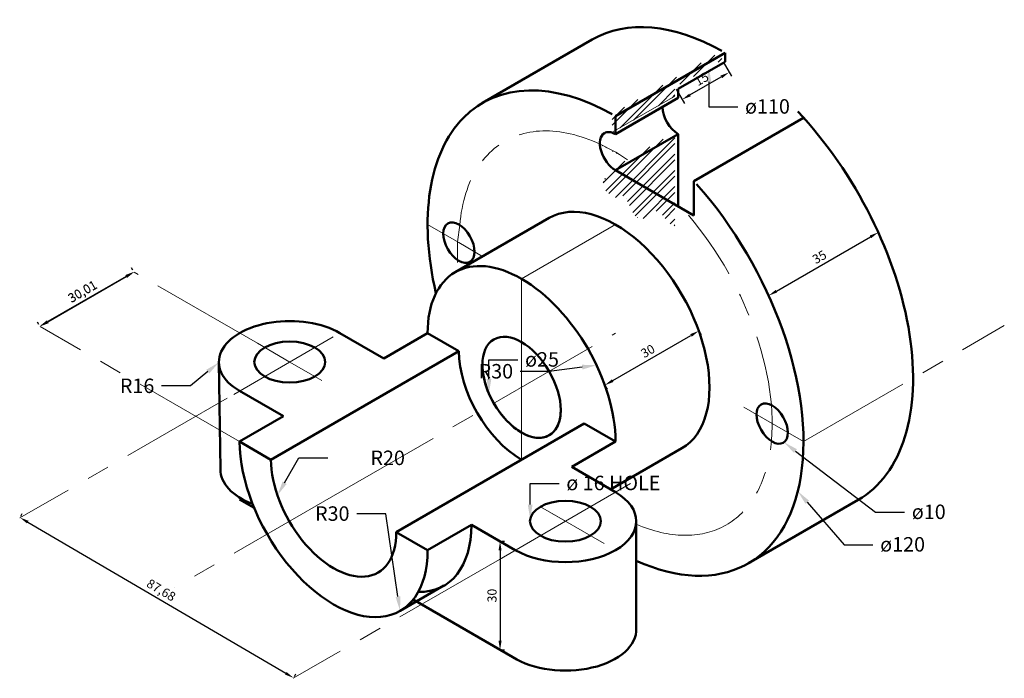
# Model space of a CAD drawing. Units: millimetres. Extents: x 2830 to 3102, y 1462 to 1644.
import ezdxf
from ezdxf import colors
from ezdxf.entities.mleader import LeaderData, LeaderLine
from ezdxf.math import Vec2, Vec3

# ---------------------------------------------------------------- set-up
doc = ezdxf.new("R2010")
doc.units = ezdxf.units.MM
doc.linetypes.add('CENTER', pattern=[50.8, 31.75, -6.35, 6.35, -6.35])
for name, color, linetype, lineweight in [('M-CNTR', 1, 'CENTER', 18), ('M-DIMS', 2, 'Continuous', 25), ('M-HATC', 8, 'Continuous', 18), ('M-OUTL', 7, 'Continuous', 50), ('M-TEXT', 3, 'Continuous', 25)]:
    doc.layers.add(name, color=color, linetype=linetype, lineweight=lineweight)
doc.styles.get("Standard").update_dxf_attribs({"font": 'arial.ttf'})
doc.dimstyles.new('ISO-25', dxfattribs={"dimtxt": 2.5, "dimasz": 2.5, "dimexe": 1.25, "dimexo": 0.625, "dimtad": 1, "dimtxsty": 'Standard', "dimcen": 2.5, "dimadec": 0, "dimazin": 0, "dimtfac": 1, "dimtmove": 0, "dimatfit": 3, "dimfxl": 1, "dimarcsym": 0})
pattern_1 = [(45, (0, 0), (-2.245064, 2.245064), []), (45, (0, 1.5875), (-2.245064, 2.245064), [])]

# ---------------------------------------------------------------- blocks, each defined once
blk = doc.blocks.new('*D1')
at = {"layer": 'Defpoints', "color": 0, "transparency": 16777216}
for p in [(2962.61, 1500.11), (2962.61, 1470.11), (2962.61, 1470.11)]:
    blk.add_point(p, dxfattribs=at)
at = {"layer": 'M-DIMS', "color": 0, "lineweight": -2, "transparency": 16777216}
for p, q in [((2963.24, 1500.11), (2963.86, 1500.11)), ((2962.61, 1497.61), (2962.61, 1472.61)), ((2963.24, 1470.11), (2963.86, 1470.11))]:
    blk.add_line(p, q, dxfattribs=at)
at = {"layer": 'M-DIMS', "color": 0, "transparency": 16777216}
for points in [[(2962.19, 1497.61), (2963.03, 1497.61), (2962.61, 1500.11)], [(2962.19, 1472.61), (2963.03, 1472.61), (2962.61, 1470.11)]]:
    blk.add_solid(points, dxfattribs=at)
at = {"layer": 'M-DIMS', "color": 0, "transparency": 16777216, "insert": (2960.71, 1485.11), "char_height": 2.5, "attachment_point": 5, "rotation": 90}
blk.add_mtext('30', dxfattribs=at)
blk = doc.blocks.new('*D2')
at = {"layer": 'Defpoints', "color": 0, "transparency": 16777216}
for p in [(3017.56, 1558.28), (3017.56, 1558.28), (2991.58, 1543.28)]:
    blk.add_point(p, dxfattribs=at)
at = {"layer": 'M-DIMS', "color": 0, "lineweight": -2, "transparency": 16777216}
for p, q in [((3017.88, 1557.74), (3018.19, 1557.2)), ((2993.75, 1544.53), (3015.4, 1557.03)), ((2991.89, 1542.74), (2992.21, 1542.2))]:
    blk.add_line(p, q, dxfattribs=at)
at = {"layer": 'M-DIMS', "color": 0, "transparency": 16777216}
for points in [[(3015.19, 1557.39), (3015.61, 1556.67), (3017.56, 1558.28)], [(2993.54, 1544.89), (2993.96, 1544.17), (2991.58, 1543.28)]]:
    blk.add_solid(points, dxfattribs=at)
at = {"layer": 'M-DIMS', "color": 0, "transparency": 16777216, "insert": (3003.62, 1552.43), "char_height": 2.5, "attachment_point": 5, "rotation": 30}
blk.add_mtext('30', dxfattribs=at)
blk = doc.blocks.new('*D3')
at = {"layer": 'Defpoints', "color": 0, "transparency": 16777216}
for p in [(3023.96, 1633.18), (3025.94, 1629.75), (3010.97, 1625.68)]:
    blk.add_point(p, dxfattribs=at)
at = {"layer": 'M-DIMS', "color": 0, "lineweight": -2, "transparency": 16777216}
for p, q in [((3024.28, 1632.64), (3026.57, 1628.66)), ((3015.12, 1623.5), (3023.78, 1628.5)), ((3011.29, 1625.14), (3013.58, 1621.16))]:
    blk.add_line(p, q, dxfattribs=at)
at = {"layer": 'M-DIMS', "color": 0, "transparency": 16777216}
for points in [[(3023.57, 1628.86), (3023.99, 1628.14), (3025.94, 1629.75)], [(3014.91, 1623.86), (3015.33, 1623.14), (3012.95, 1622.25)]]:
    blk.add_solid(points, dxfattribs=at)
at = {"layer": 'M-DIMS', "color": 0, "transparency": 16777216, "insert": (3018.5, 1627.64), "char_height": 2.5, "attachment_point": 5, "rotation": 30}
blk.add_mtext('15', dxfattribs=at)
blk = doc.blocks.new('*D4')
at = {"layer": 'Defpoints', "color": 0, "transparency": 16777216}
for p in [(3067.18, 1585.53), (3067.18, 1585.53), (3036.87, 1568.03)]:
    blk.add_point(p, dxfattribs=at)
at = {"layer": 'M-DIMS', "color": 0, "lineweight": -2, "transparency": 16777216}
for p, q in [((3067.49, 1584.99), (3067.81, 1584.45)), ((3039.03, 1569.28), (3065.02, 1584.28)), ((3037.18, 1567.49), (3037.49, 1566.95))]:
    blk.add_line(p, q, dxfattribs=at)
at = {"layer": 'M-DIMS', "color": 0, "transparency": 16777216}
for points in [[(3064.81, 1584.64), (3065.22, 1583.92), (3067.18, 1585.53)], [(3038.83, 1569.64), (3039.24, 1568.92), (3036.87, 1568.03)]]:
    blk.add_solid(points, dxfattribs=at)
at = {"layer": 'M-DIMS', "color": 0, "transparency": 16777216, "insert": (3051.07, 1578.43), "char_height": 2.5, "attachment_point": 5, "rotation": 30}
blk.add_mtext('35', dxfattribs=at)
blk = doc.blocks.new('*D5')
at = {"layer": 'Defpoints', "color": 0, "transparency": 16777216}
for p in [(2829.8, 1506.56), (2905.45, 1462.24), (2905.52, 1462.36)]:
    blk.add_point(p, dxfattribs=at)
at = {"layer": 'M-DIMS', "color": 0, "lineweight": -2, "transparency": 16777216}
for p, q in [((2830.12, 1507.1), (2830.5, 1507.76)), ((2832.03, 1505.42), (2903.37, 1463.63)), ((2905.77, 1462.78), (2906.16, 1463.44))]:
    blk.add_line(p, q, dxfattribs=at)
at = {"layer": 'M-DIMS', "color": 0, "transparency": 16777216}
for points in [[(2832.24, 1505.78), (2831.82, 1505.06), (2829.87, 1506.69)], [(2903.58, 1463.99), (2903.16, 1463.27), (2905.52, 1462.36)]]:
    blk.add_solid(points, dxfattribs=at)
at = {"layer": 'M-DIMS', "color": 0, "transparency": 16777216, "insert": (2868.77, 1486.36), "char_height": 2.5, "attachment_point": 5, "rotation": 329.6353}
blk.add_mtext('87,68', dxfattribs=at)
blk = doc.blocks.new('*D6')
at = {"layer": 'Defpoints', "color": 0, "transparency": 16777216}
for p in [(2829.8, 1506.56), (2905.45, 1462.24), (2905.52, 1462.36)]:
    blk.add_point(p, dxfattribs=at)
at = {"layer": 'M-DIMS', "color": 0, "lineweight": -2, "transparency": 16777216}
for p, q in [((2830.12, 1507.1), (2830.5, 1507.76)), ((2832.03, 1505.42), (2903.37, 1463.63)), ((2905.77, 1462.78), (2906.16, 1463.44))]:
    blk.add_line(p, q, dxfattribs=at)
at = {"layer": 'M-DIMS', "color": 0, "transparency": 16777216}
for points in [[(2832.24, 1505.78), (2831.82, 1505.06), (2829.87, 1506.69)], [(2903.58, 1463.99), (2903.16, 1463.27), (2905.52, 1462.36)]]:
    blk.add_solid(points, dxfattribs=at)
at = {"layer": 'M-DIMS', "color": 0, "transparency": 16777216, "insert": (2868.77, 1486.36), "char_height": 2.5, "attachment_point": 5, "rotation": 329.6353}
blk.add_mtext('87,68', dxfattribs=at)
blk = doc.blocks.new('*D7')
at = {"layer": 'Defpoints', "color": 0, "transparency": 16777216}
for p in [(2861.42, 1574.53), (2835.38, 1559.61), (2835.43, 1559.53)]:
    blk.add_point(p, dxfattribs=at)
at = {"layer": 'M-DIMS', "color": 0, "lineweight": -2, "transparency": 16777216}
for p, q in [((2861.1, 1575.08), (2860.74, 1575.7)), ((2859.2, 1573.36), (2837.55, 1560.86)), ((2835.11, 1560.07), (2834.76, 1560.69))]:
    blk.add_line(p, q, dxfattribs=at)
at = {"layer": 'M-DIMS', "color": 0, "transparency": 16777216}
for points in [[(2859, 1573.72), (2859.41, 1573), (2861.37, 1574.61)], [(2837.34, 1561.22), (2837.76, 1560.5), (2835.38, 1559.61)]]:
    blk.add_solid(points, dxfattribs=at)
at = {"layer": 'M-DIMS', "color": 0, "transparency": 16777216, "insert": (2847.31, 1568.95), "char_height": 2.5, "attachment_point": 5, "rotation": 30}
blk.add_mtext('30,01', dxfattribs=at)
blk = doc.blocks.new('*D8')
at = {"layer": 'Defpoints', "color": 0, "transparency": 16777216}
for p in [(2861.42, 1574.53), (2861.42, 1574.53), (2835.43, 1559.53)]:
    blk.add_point(p, dxfattribs=at)
at = {"layer": 'M-DIMS', "color": 0, "lineweight": -2, "transparency": 16777216}
for p, q in [((2861.1, 1575.08), (2860.79, 1575.62)), ((2837.59, 1560.78), (2859.25, 1573.28)), ((2835.11, 1560.07), (2834.8, 1560.61))]:
    blk.add_line(p, q, dxfattribs=at)
at = {"layer": 'M-DIMS', "color": 0, "transparency": 16777216}
for points in [[(2859.04, 1573.65), (2859.46, 1572.92), (2861.42, 1574.53)], [(2837.38, 1561.14), (2837.8, 1560.42), (2835.43, 1559.53)]]:
    blk.add_solid(points, dxfattribs=at)
at = {"layer": 'M-DIMS', "color": 0, "transparency": 16777216, "insert": (2847.36, 1568.87), "char_height": 2.5, "attachment_point": 5, "rotation": 30}
blk.add_mtext('30,01', dxfattribs=at)

msp = doc.modelspace()

# ---------------------------------------------------------------- hatches: boundary and pattern name
at = {"layer": 'M-HATC'}
h = msp.add_hatch(dxfattribs=at)
h.set_pattern_fill('STEEL', color=256)
h.set_pattern_definition(pattern_1)
h.paths.add_polyline_path([(3010.973, 1623.178), (3010.973, 1625.678), (3023.963, 1633.178), (3023.963, 1635.679), (2993.652, 1618.179), (2993.652, 1613.177)])
h = msp.add_hatch(dxfattribs=at)
h.set_pattern_fill('STEEL', color=256)
h.set_pattern_definition(pattern_1)
h.paths.add_polyline_path([(2996.27, 1595.472), (2996.241, 1595.455), (2996.172, 1595.411), (2996.221, 1595.442)])
h.paths.add_polyline_path([(3006.737, 1619.58), (3006.744, 1619.541), (3006.74, 1619.567), (3006.735, 1619.593), (3006.731, 1619.619)])
h.paths.add_polyline_path([(2996.46, 1595.577), (2996.438, 1595.567), (2996.413, 1595.554)])
h.paths.add_polyline_path([(2996.552, 1595.616), (2996.531, 1595.609), (2996.506, 1595.598)])
h.paths.add_polyline_path([(3006.721, 1619.684), (3006.727, 1619.645), (3006.723, 1619.671), (3006.719, 1619.697), (3006.715, 1619.723)])
h.paths.add_polyline_path([(3006.755, 1619.476), (3006.763, 1619.436), (3006.758, 1619.462), (3006.753, 1619.489), (3006.749, 1619.515)])
h.paths.add_polyline_path([(2996.366, 1595.528), (2996.345, 1595.517), (2996.318, 1595.501)])
h.paths.add_polyline_path([(2996.643, 1595.643), (2996.622, 1595.639), (2996.598, 1595.631)])
h.paths.add_polyline_path([(3006.706, 1619.788), (3006.711, 1619.749), (3006.708, 1619.775), (3006.704, 1619.801), (3006.701, 1619.827)])
h.paths.add_polyline_path([(3006.775, 1619.37), (3006.783, 1619.331), (3006.778, 1619.357), (3006.773, 1619.384), (3006.768, 1619.41)])
h.paths.add_polyline_path([(3006.692, 1619.891), (3006.697, 1619.852), (3006.694, 1619.878), (3006.691, 1619.904), (3006.688, 1619.929)])
h.paths.add_polyline_path([(2996.734, 1595.655), (2996.712, 1595.655), (2996.689, 1595.651)])
h.paths.add_polyline_path([(3006.68, 1619.993), (3006.685, 1619.955), (3006.682, 1619.981), (3006.679, 1620.006), (3006.677, 1620.032)])
h.paths.add_polyline_path([(3006.797, 1619.265), (3006.805, 1619.225), (3006.8, 1619.252), (3006.794, 1619.278), (3006.789, 1619.304)])
h.paths.add_polyline_path([(3006.67, 1620.095), (3006.674, 1620.057), (3006.671, 1620.082), (3006.669, 1620.108), (3006.667, 1620.133)])
h.paths.add_polyline_path([(2996.824, 1595.65), (2996.802, 1595.655), (2996.779, 1595.655)])
h.paths.add_polyline_path([(3006.661, 1620.196), (3006.665, 1620.158), (3006.663, 1620.183), (3006.661, 1620.209), (3006.659, 1620.234)])
h.paths.add_polyline_path([(3006.819, 1619.159), (3006.829, 1619.119), (3006.823, 1619.146), (3006.817, 1619.172), (3006.811, 1619.199)])
h.paths.add_polyline_path([(3006.654, 1620.296), (3006.657, 1620.259), (3006.655, 1620.284), (3006.654, 1620.309), (3006.652, 1620.334)])
h.paths.add_polyline_path([(2996.913, 1595.625), (2996.892, 1595.635), (2996.869, 1595.64)])
h.paths.add_polyline_path([(3006.649, 1620.396), (3006.651, 1620.358), (3006.65, 1620.383), (3006.649, 1620.408), (3006.648, 1620.433)])
h.paths.add_polyline_path([(3006.843, 1619.057), (3006.847, 1619.039), (3006.841, 1619.066), (3006.835, 1619.092)])
h.paths.add_polyline_path([(3006.645, 1620.494), (3006.647, 1620.457), (3006.646, 1620.482), (3006.645, 1620.507), (3006.644, 1620.531)])
h.paths.add_polyline_path([(2997.003, 1595.579), (2996.981, 1595.595), (2996.958, 1595.605)])
h.paths.add_polyline_path([(3006.643, 1620.592), (3006.644, 1620.555), (3006.643, 1620.58), (3006.643, 1620.604), (3006.643, 1620.628)])
h.paths.add_polyline_path([(2997.094, 1595.508), (2997.072, 1595.53), (2997.049, 1595.547)])
h.paths.add_polyline_path([(3006.642, 1620.677), (3006.643, 1620.653), (3006.642, 1620.677)])
h.paths.add_polyline_path([(2997.185, 1595.411), (2997.162, 1595.44), (2997.139, 1595.463)])
h = msp.add_hatch(dxfattribs=at)
h.set_pattern_fill('STARS', color=256)
edge = h.paths.add_edge_path(flags=17)
edge.add_line((3010.973, 1613.177), (2997.982, 1605.677))
edge.add_ellipse((2993.652, 1608.177), major_axis=(3.062, -5.303), ratio=0.5773503, start_angle=28.55472, end_angle=30, ccw=False)
edge.add_ellipse((2994.538, 1557.676), major_axis=(30.619, -53.033), ratio=0.5773503, start_angle=146.03159, end_angle=155.64724, ccw=False)
edge.add_line((2997.863, 1605.608), (2993.652, 1603.177))
edge.add_spline(control_points=[(2993.652, 1603.177), (2989.631, 1598.94), (2992.844, 1596.003), (2995.663, 1594.375), (2997.082, 1596.832), (2998.786, 1591.134), (3001.829, 1587.953), (3006.458, 1593.12), (3008.118, 1588.818), (3010.248, 1587.415), (3010.973, 1587.275)], knot_values=[0, 0, 0, 0, 1, 2, 3, 4, 5, 6, 7, 7.4719642, 7.4719642, 7.4719642, 7.4719642], degree=3, periodic=0)
edge.add_line((3010.973, 1587.275), (3010.973, 1613.177))
edge = h.paths.add_edge_path(flags=17)
edge.add_line((3010.973, 1613.177), (2997.982, 1605.677))
edge.add_ellipse((2993.652, 1608.177), major_axis=(3.062, -5.303), ratio=0.5773503, start_angle=29.2721, end_angle=30, ccw=False)
edge.add_ellipse((2994.538, 1557.676), major_axis=(30.619, -53.033), ratio=0.5773503, start_angle=146.03159, end_angle=155.64724, ccw=False)
edge.add_line((2997.863, 1605.608), (2993.652, 1603.177))
edge.add_line((2993.652, 1603.177), (2991.105, 1598.999))
edge.add_line((2991.105, 1598.999), (2992.044, 1596.855))
edge.add_line((2992.044, 1596.855), (2993.629, 1595.653))
edge.add_line((2993.629, 1595.653), (2994.875, 1595.072))
edge.add_line((2994.875, 1595.072), (2995.823, 1595.202))
edge.add_line((2995.823, 1595.202), (2995.963, 1595.281))
edge.add_spline(control_points=[(2995.963, 1595.281), (2996.181, 1595.411), (2996.378, 1595.557), (2996.568, 1595.622)], knot_values=[2.2737758, 2.2737758, 2.2737758, 2.2737758, 2.6371638, 2.6371638, 2.6371638, 2.6371638], degree=3, periodic=0)
edge.add_line((2996.534, 1595.637), (2996.568, 1595.622))
edge.add_spline(control_points=[(2996.568, 1595.622), (2996.758, 1595.686), (2996.979, 1595.665), (2997.21, 1595.382), (2997.25, 1595.326)], knot_values=[2.6371638, 2.6371638, 2.6371638, 2.6371638, 3, 3.0766912, 3.0766912, 3.0766912, 3.0766912], degree=3, periodic=0)
edge.add_spline(control_points=[(2997.25, 1595.326), (2997.483, 1595.001), (2997.727, 1594.44), (2997.998, 1593.794)], knot_values=[3.0766912, 3.0766912, 3.0766912, 3.0766912, 3.5162185, 3.5162185, 3.5162185, 3.5162185], degree=3, periodic=0)
edge.add_line((2997.998, 1593.794), (2998.905, 1591.752))
edge.add_line((2998.905, 1591.752), (3000.054, 1590.055))
edge.add_line((3000.054, 1590.055), (3001.481, 1589.29))
edge.add_line((3001.481, 1589.29), (3003.191, 1589.866))
edge.add_line((3003.191, 1589.866), (3003.643, 1590.164))
edge.add_spline(control_points=[(3003.643, 1590.164), (3004.098, 1590.474), (3004.552, 1590.805), (3004.981, 1591.044)], knot_values=[5.3837355, 5.3837355, 5.3837355, 5.3837355, 5.713855, 5.713855, 5.713855, 5.713855], degree=3, periodic=0)
edge.add_spline(control_points=[(3004.981, 1591.044), (3005.353, 1591.252), (3005.895, 1591.466), (3006.352, 1591.345), (3006.505, 1591.27)], knot_values=[5.713855, 5.713855, 5.713855, 5.713855, 6, 6.1533823, 6.1533823, 6.1533823, 6.1533823], degree=3, periodic=0)
edge.add_spline(control_points=[(3006.505, 1591.27), (3006.943, 1591.056), (3007.325, 1590.575), (3007.733, 1590.019)], knot_values=[6.1533823, 6.1533823, 6.1533823, 6.1533823, 6.5929096, 6.5929096, 6.5929096, 6.5929096], degree=3, periodic=0)
edge.add_line((3007.733, 1590.019), (3009.118, 1588.318))
edge.add_line((3009.118, 1588.318), (3010.973, 1587.275))
edge.add_line((3010.973, 1587.275), (3010.973, 1613.177))
h = msp.add_hatch(dxfattribs=at)
h.set_pattern_fill('STEEL', color=256)
h.set_pattern_definition(pattern_1)
edge = h.paths.add_edge_path()
edge.add_line((3010.973, 1613.177), (2997.982, 1605.677))
edge.add_ellipse((2993.652, 1608.177), major_axis=(3.062, -5.303), ratio=0.5773503, start_angle=28.55472, end_angle=30, ccw=False)
edge.add_ellipse((2994.538, 1557.676), major_axis=(30.619, -53.033), ratio=0.5773503, start_angle=146.03159, end_angle=155.64724, ccw=False)
edge.add_line((2997.863, 1605.608), (2993.652, 1603.177))
edge.add_spline(control_points=[(2993.652, 1603.177), (2989.631, 1598.94), (2992.844, 1596.003), (2995.663, 1594.375), (2997.082, 1596.832), (2998.786, 1591.134), (3001.829, 1587.953), (3006.458, 1593.12), (3008.118, 1588.818), (3010.248, 1587.415), (3010.973, 1587.275)], knot_values=[0, 0, 0, 0, 1, 2, 3, 4, 5, 6, 7, 7.4719642, 7.4719642, 7.4719642, 7.4719642], degree=3, periodic=0)
edge.add_line((3010.973, 1587.275), (3010.973, 1613.177))

# ---------------------------------------------------------------- linework, layer by layer
at = {"layer": 'M-CNTR'}
for p, q in [((3006.642, 1620.677), (3010.973, 1623.177)), ((2993.652, 1613.177), (3006.642, 1620.677)), ((2951.237, 1582.676), (2942.577, 1587.676)), ((2951.453, 1587.544), (2950.83, 1582.911)), ((2968.557, 1572.676), (2994.538, 1587.676)), ((2950.83, 1582.911), (2950.83, 1577.172)), ((2951.237, 1582.676), (2957.796, 1578.889)), ((2895.512, 1554.848), (2861.415, 1574.534)), ((2968.557, 1542.676), (2968.557, 1572.676)), ((2890.615, 1527.668), (2835.427, 1559.53)), ((2916.596, 1512.676), (2994.538, 1557.676)), ((3046.5, 1527.676), (3102.024, 1559.733)), ((2916.494, 1556.617), (2887.186, 1539.696)), ((2904.472, 1549.676), (2895.512, 1554.848)), ((2911.4, 1545.676), (2904.472, 1549.676)), ((2911.4, 1545.676), (2913.291, 1544.584)), ((2968.557, 1542.676), (2968.557, 1522.676)), ((2887.186, 1539.696), (2829.801, 1506.565)), ((3037.839, 1532.676), (3030.05, 1537.173)), ((3037.839, 1532.676), (3046.5, 1527.676)), ((2980.682, 1505.676), (2998.697, 1516.077)), ((2916.596, 1512.676), (2872.583, 1487.265)), ((2973.754, 1509.676), (2980.682, 1505.676)), ((2973.754, 1509.676), (2991.349, 1499.517)), ((2980.682, 1505.676), (2962.415, 1495.129)), ((2962.415, 1495.129), (2905.454, 1462.243))]:
    msp.add_line(p, q, dxfattribs=at)
for start_param, end_param in [(2.2793263, 3.8269491), (5.6294391, 8.1539794)]:
    msp.add_ellipse((2994.538, 1557.676), major_axis=(30.619, -53.033), ratio=0.5773503, start_param=start_param, end_param=end_param, dxfattribs=at)
at = {"layer": 'M-OUTL'}
for p, q in [((2957.796, 1621.315), (2988.107, 1638.815)), ((2988.107, 1638.815), (2957.796, 1621.315)), ((2994.538, 1617.676), (3024.849, 1635.176)), ((3024.849, 1632.676), (3024.849, 1635.176)), ((3011.859, 1625.176), (3024.849, 1632.676)), ((3011.859, 1625.176), (3011.859, 1622.676)), ((2994.538, 1612.676), (3011.859, 1622.676)), ((2994.538, 1617.676), (2994.538, 1612.676)), ((3016.189, 1599.72), (3046.5, 1617.22)), ((2994.538, 1602.676), (3011.859, 1612.676)), ((3011.859, 1612.676), (3011.859, 1592.676)), ((3016.189, 1590.176), (2994.538, 1602.676)), ((3016.189, 1599.72), (3016.189, 1590.176)), ((2950.186, 1574.495), (2976.167, 1589.495)), ((2918.328, 1557.676), (2930.452, 1550.676)), ((2930.452, 1550.676), (2942.577, 1557.676)), ((2951.237, 1552.676), (2942.577, 1557.676)), ((2899.275, 1522.676), (2951.237, 1552.676)), ((2899.275, 1522.676), (2951.237, 1552.676)), ((2885.305, 1520.062), (2884.876, 1549.581)), ((2890.615, 1541.676), (2902.74, 1534.676)), ((2890.615, 1527.676), (2902.74, 1534.676)), ((2933.916, 1502.676), (2985.878, 1532.676)), ((2985.878, 1532.676), (2994.538, 1527.676)), ((2899.275, 1522.676), (2890.615, 1527.676)), ((2982.414, 1520.676), (2994.538, 1527.676)), ((2982.414, 1520.676), (2994.538, 1527.676)), ((3012.909, 1525.856), (2993.175, 1514.462)), ((2982.414, 1520.676), (2994.538, 1513.676)), ((2894.619, 1509.365), (2890.615, 1511.676)), ((3031.281, 1494.036), (3061.591, 1511.536)), ((3000.278, 1475.676), (3000.278, 1505.676)), ((2933.916, 1502.676), (2942.577, 1497.676)), ((2942.577, 1497.676), (2933.916, 1502.676)), ((2942.577, 1497.676), (2954.701, 1504.676)), ((2942.577, 1497.676), (2954.701, 1504.676)), ((2954.701, 1504.676), (2966.825, 1497.676)), ((2934.967, 1480.856), (2947.092, 1487.856)), ((2966.144, 1468.089), (2938.584, 1484.001))]:
    msp.add_line(p, q, dxfattribs=at)
for centre, major_axis, start_param, end_param in [((3024.849, 1575.176), (36.742, -63.64), 2.3732487, 3.1415927), ((2994.538, 1557.676), (36.742, -63.64), 8.656434, 10.5088793), ((3011.859, 1617.676), (3.062, -5.303), 3.9269908, 5.4977871), ((3024.849, 1575.176), (36.742, -63.64), 0, 1.9596753), ((2994.538, 1607.676), (3.062, -5.303), 3.1415927, 5.4977871), ((2994.538, 1607.676), (3.062, -5.303), 2.3561945, 3.1415927), ((2994.538, 1557.676), (36.742, -63.64), 5.6084699, 8.1933451), ((2994.538, 1557.676), (18.371, -31.82), 0, 3.1415927), ((2968.558, 1542.676), (18.371, -31.82), 2.3561945, 3.1415927), ((2968.558, 1542.676), (18.371, -31.82), 3.1415927, 3.9269908), ((2994.538, 1557.676), (30.619, -53.033), 4.0688879, 4.0712043), ((2968.558, 1542.676), (18.371, -31.82), 0.7853982, 2.3561945), ((2904.472, 1549.676), (-19.596, 0), 3.9269908, 7.0685835), ((2968.557, 1542.676), (12.247, -21.213), 3.9269908, 5.4977871), ((2968.557, 1542.676), (7.655, -13.258), 3.9269908, 7.0685835), ((2904.899, 1519.923), (-19.596, 0), 5.4977871, 5.5291568), ((2916.596, 1512.676), (18.371, -31.82), 3.9269908, 7.0685835), ((2916.596, 1512.676), (12.247, -21.213), 3.9269908, 7.0685835), ((2904.899, 1519.923), (-19.596, 0), 6.2708926, 7.2751503), ((2980.682, 1505.676), (-19.596, 0), 0.7853982, 3.9269908), ((2928.72, 1519.676), (18.371, -31.82), 5.9468996, 7.0685835), ((2980.682, 1475.676), (-19.596, 0), 0.7349544, 3.1742786)]:
    msp.add_ellipse(centre, major_axis=major_axis, ratio=0.5773503, start_param=start_param, end_param=end_param, dxfattribs=at)
for centre, major_axis in [((2951.237, 1582.676), (3.062, -5.303)), ((2968.557, 1542.676), (7.655, -13.258)), ((2904.472, 1549.676), (-9.798, 0)), ((3037.839, 1532.676), (3.062, -5.303)), ((2980.682, 1505.676), (-9.798, 0))]:
    msp.add_ellipse(centre, major_axis=major_axis, ratio=0.5773503, dxfattribs=at)

# ---------------------------------------------------------------- dimensions: what is measured, and where the dimension line sits
at = {"layer": 'M-DIMS'}
for p1, p2, distance, picture, middle in [((3010.973, 1625.678), (3023.963, 1633.178), -3.963, '*D3', (3018.499, 1627.643)), ((3036.87, 1568.031), (3067.18, 1585.531), 0, '*D4', (3051.074, 1578.429)), ((2991.582, 1543.28), (3017.563, 1558.28), 0, '*D2', (3003.621, 1552.428)), ((2962.611, 1500.109), (2962.611, 1470.109), 0, '*D1', (2960.709, 1485.109))]:
    dim = msp.add_aligned_dim(p1=p1, p2=p2, distance=distance, dimstyle='ISO-25', override={"dimclrd": 0, "dimclre": 0, "dimclrt": 0}, dxfattribs=at)
    dim.commit()
    dim.dimension.update_dxf_attribs({"geometry": picture, "text_midpoint": middle})
for base, p1, p2, angle, picture, middle in [((2835.382, 1559.61), (2861.415, 1574.534), (2835.427, 1559.53), 210, '*D7', (2847.312, 1568.954)), ((2861.415, 1574.534), (2835.427, 1559.53), (2861.415, 1574.534), 30, '*D8', (2847.358, 1568.875)), ((2905.524, 1462.363), (2829.801, 1506.565), (2905.454, 1462.243), 329.63528, '*D5', (2868.774, 1486.36)), ((2905.524, 1462.363), (2829.801, 1506.565), (2905.454, 1462.243), 329.63528, '*D6', (2868.774, 1486.36))]:
    dim = msp.add_linear_dim(base=base, p1=p1, p2=p2, angle=angle, dimstyle='ISO-25', override={"dimrnd": 0}, dxfattribs=at)
    dim.commit()
    dim.dimension.update_dxf_attribs({"geometry": picture, "text_midpoint": middle})

# ---------------------------------------------------------------- leaders
at = {"layer": 'M-TEXT'}
ml = msp.add_multileader_mtext('Standard', dxfattribs=at)
ml.set_content('ø110', color=256)
ml.set_leader_properties()
ml.build(insert=Vec2(0, 0))
ctx = ml.context
ctx.base_point, ctx.plane_origin = Vec3(3028.354, 1620.233), Vec3(3020.354, 1631.095)
notes = []
notes.append((ctx, [(0, (1, 1, 0), (3020.354, 1620.233), (1, 0), 8, [(0, [(3020.354, 1631.095)], 0, [])])]))
ctx.mtext.insert, ctx.mtext.flow_direction = Vec3(3030.354, 1622.341), 5
ml = msp.add_multileader_mtext('Standard', dxfattribs=at)
ml.set_content('ø25', color=256)
ml.set_leader_properties()
ml.build(insert=Vec2(0, 0))
ctx = ml.context
ctx.base_point, ctx.plane_origin = Vec3(2967.535, 1550.293), Vec3(2959.535, 1540.977)
notes.append((ctx, [(0, (1, 1, 0), (2959.535, 1550.293), (1, 0), 8, [(0, [(2959.535, 1540.977)], 0, [])])]))
ctx.mtext.insert, ctx.mtext.flow_direction = Vec3(2969.535, 1552.401), 5
ml = msp.add_multileader_mtext('Standard', dxfattribs=at)
ml.set_content('R16', color=256)
ml.set_leader_properties()
ml.build(insert=Vec2(0, 0))
ctx = ml.context
ctx.base_point, ctx.plane_origin = Vec3(2855.471, 1543.075), Vec3(2884.876, 1549.581)
ctx.text_align_type = 2
notes.append((ctx, [(0, (1, 1, 0), (2877.026, 1543.075), (-1, 0), 8, [(0, [(2884.876, 1549.581)], 0, [])])]))
ctx.mtext.insert, ctx.mtext.alignment, ctx.mtext.flow_direction = Vec3(2867.026, 1545.109), 3, 5
ml = msp.add_multileader_mtext('Standard', dxfattribs=at)
ml.set_content('R30', color=256)
ml.set_leader_properties()
ml.build(insert=Vec2(0, 0))
ctx = ml.context
ctx.base_point, ctx.plane_origin = Vec3(2954.668, 1547.095), Vec3(2989.289, 1548.787)
ctx.text_align_type = 2
notes.append((ctx, [(0, (1, 1, 0), (2976.212, 1547.095), (-1, 0), 8, [(0, [(2989.289, 1548.787)], 0, [])])]))
ctx.mtext.insert, ctx.mtext.alignment, ctx.mtext.flow_direction = Vec3(2966.212, 1549.131), 3, 5
ml = msp.add_multileader_mtext('Standard', dxfattribs=at)
ml.set_content('ø10', color=256)
ml.set_leader_properties()
ml.build(insert=Vec2(0, 0))
ctx = ml.context
ctx.base_point, ctx.plane_origin = Vec3(3074.457, 1508.165), Vec3(3041.098, 1527.501)
notes.append((ctx, [(0, (1, 1, 0), (3066.457, 1508.165), (1, 0), 8, [(0, [(3041.098, 1527.501)], 0, [])])]))
ctx.mtext.insert, ctx.mtext.flow_direction = Vec3(3076.457, 1510.273), 5
ml = msp.add_multileader_mtext('Standard', dxfattribs=at)
ml.set_content('^IR20', color=256)
ml.set_leader_properties()
ml.build(insert=Vec2(0, 0))
ctx = ml.context
ctx.base_point, ctx.plane_origin = Vec3(2915.008, 1523.156), Vec3(2901.049, 1512.836)
notes.append((ctx, [(0, (1, 1, 0), (2907.008, 1523.156), (1, 0), 8, [(0, [(2901.049, 1512.836)], 0, [])])]))
ctx.mtext.insert, ctx.mtext.flow_direction = Vec3(2917.008, 1525.19), 5
ml = msp.add_multileader_mtext('Standard', dxfattribs=at)
ml.set_content('ø 16 HOLE', color=256)
ml.set_leader_properties()
ml.build(insert=Vec2(0, 0))
ctx = ml.context
ctx.base_point, ctx.plane_origin = Vec3(2978.937, 1516.135), Vec3(2970.937, 1506.265)
notes.append((ctx, [(0, (1, 1, 0), (2970.937, 1516.135), (1, 0), 8, [(0, [(2970.937, 1506.265)], 0, [])])]))
ctx.mtext.insert, ctx.mtext.flow_direction = Vec3(2980.937, 1518.243), 5
ml = msp.add_multileader_mtext('Standard', dxfattribs=at)
ml.set_content('ø120', color=256)
ml.set_leader_properties()
ml.build(insert=Vec2(0, 0))
ctx = ml.context
ctx.base_point, ctx.plane_origin = Vec3(3065.713, 1499.172), Vec3(3044.929, 1513.942)
notes.append((ctx, [(0, (1, 1, 0), (3057.713, 1499.172), (1, 0), 8, [(0, [(3044.929, 1513.942)], 0, [])])]))
ctx.mtext.insert, ctx.mtext.flow_direction = Vec3(3067.713, 1501.28), 5
ml = msp.add_multileader_mtext('Standard', dxfattribs=at)
ml.set_content('R30', color=256)
ml.set_leader_properties()
ml.build(insert=Vec2(0, 0))
ctx = ml.context
ctx.base_point, ctx.plane_origin = Vec3(2909.443, 1507.75), Vec3(2934.967, 1480.856)
ctx.text_align_type = 2
notes.append((ctx, [(0, (1, 1, 0), (2930.987, 1507.75), (-1, 0), 8, [(0, [(2934.967, 1480.856)], 0, [])])]))
ctx.mtext.insert, ctx.mtext.alignment, ctx.mtext.flow_direction = Vec3(2920.987, 1509.785), 3, 5
for ctx, leaders in notes:
    for number, flags, end, landing, length, lines in leaders:
        leader = LeaderData()
        leader.index, (leader.has_last_leader_line, leader.has_dogleg_vector, leader.attachment_direction) = number, flags
        leader.last_leader_point, leader.dogleg_vector, leader.dogleg_length = Vec3(end), Vec3(landing), length
        for number, points, colour, breaks in lines:
            line = LeaderLine()
            line.index, line.vertices, line.color, line.breaks = number, Vec3.list(points), colors.encode_raw_color(colour), breaks
            leader.lines.append(line)
        ctx.leaders.append(leader)

doc.saveas('drawing.dxf')
